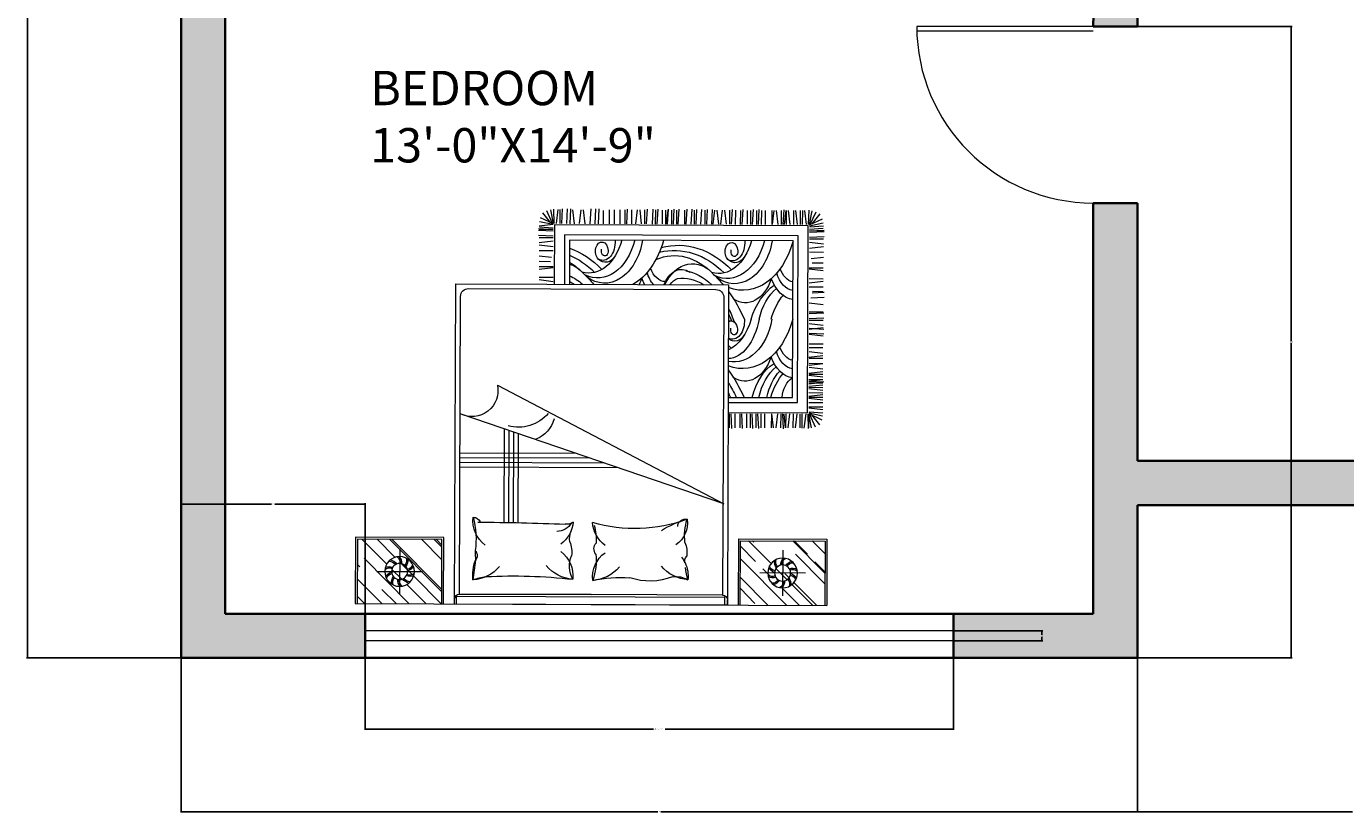
# Model space of a CAD drawing. Units: inches. Extents: x 1919 to 2461, y 2470 to 3159.
# Tile 1 of 6: x 1919 to 2188, y 2470 to 2630. Entities that reach past the tile are written whole.
import ezdxf

# ---------------------------------------------------------------- set-up
doc = ezdxf.new("R2010")
doc.units = ezdxf.units.IN
for name, color, linetype, lineweight in [('A-ANNO-DIMS', 2, 'Continuous', 18), ('A-AREA-IDEN', 7, 'Continuous', 18), ('A-DOOR', 3, 'Continuous', 18), ('A-FURN', 8, 'Continuous', 18), ('A-GLAZ', 4, 'Continuous', 18), ('A-WALL', 7, 'Continuous', 35), ('A-WALL-PATT', 252, 'Continuous', 13)]:
    doc.layers.add(name, color=color, linetype=linetype, lineweight=lineweight)
doc.styles.get("Standard").update_dxf_attribs({"font": 'arial.ttf'})
doc.dimstyles.get("Standard").update_dxf_attribs({"dimtxt": 0.18, "dimasz": 0.18, "dimexe": 0.18, "dimexo": 0.0625, "dimgap": 0.09, "dimtad": 0, "dimtih": 1, "dimtoh": 1, "dimdec": 4, "dimzin": 0, "dimdsep": 46, "dimtxsty": 'Standard', "dimcen": 0.09, "dimadec": 0, "dimazin": 0, "dimtfac": 1, "dimtdec": 4, "dimtofl": 0, "dimtmove": 0, "dimatfit": 3, "dimfxl": 1, "dimtolj": 1, "dimtzin": 0, "dimarcsym": 0})

# ---------------------------------------------------------------- blocks, each defined once
blk = doc.blocks.new('A$C64B41DC1')
for p, q in [((0, 2.5079), (2.9903, 2.5079)), ((0, 2.0879), (0, 2.5079)), ((0.012, 2.4618), (0.0581, 2.5079)), ((0.012, 2.3515), (0.1684, 2.5079)), ((0.012, 2.0999), (0.012, 2.5079)), ((0.0543, 2.2213), (0.3409, 2.5079)), ((0.1689, 2.4179), (0.2589, 2.5079)), ((0.2157, 2.0999), (0.548, 2.4322)), ((0.2804, 2.1597), (0.2804, 2.4481)), ((0.3265, 2.386), (0.4484, 2.5079)), ((0.3699, 2.3332), (0.5445, 2.5079)), ((0.548, 2.5079), (0.548, 2.0999)), ((0.56, 2.5079), (0.56, 2.0879)), ((0.6301, 2.5079), (0.6301, 0.4779)), ((0.6401, 2.461), (0.6401, 2.5079)), ((0.6401, 2.5079), (2.344, 2.5079)), ((2.344, 2.461), (0.6401, 2.461)), ((0.6601, 2.4461), (1.4951, 2.4461)), ((0.6601, 2.4461), (0.6601, 0.5579)), ((1.4951, 2.4461), (0.6697, 2.4461)), ((2.3301, 2.4461), (1.4951, 2.4461)), ((2.3301, 0.5579), (2.3301, 2.4461)), ((2.344, 2.5079), (2.3601, 2.5079)), ((2.344, 2.5079), (2.344, 2.461)), ((2.3601, 2.5079), (2.3601, 2.4761)), ((2.3601, 0.4779), (2.3601, 2.5079)), ((2.4303, 2.5079), (2.4303, 2.0879)), ((2.4423, 2.5079), (2.4423, 2.0999)), ((2.4423, 2.3333), (2.6169, 2.5079)), ((2.4423, 2.2145), (2.7357, 2.5079)), ((2.4423, 2.404), (2.5354, 2.4971)), ((2.705, 2.398), (2.8149, 2.5079)), ((2.7099, 2.1597), (2.7099, 2.4481)), ((2.7691, 2.3772), (2.8998, 2.5079)), ((2.7819, 2.3646), (2.9252, 2.5079)), ((2.9783, 2.0999), (2.9783, 2.5079)), ((2.9903, 2.0879), (2.9903, 2.5079)), ((0.2299, 2.0999), (0.548, 2.418)), ((0.2311, 2.2906), (0.2937, 2.3532)), ((2.6674, 2.2756), (2.7382, 2.3464)), ((2.7914, 2.1846), (2.9783, 2.3715)), ((0.012, 2.261), (0.0275, 2.2765)), ((0.1362, 2.3039), (0.4246, 2.3039)), ((0.2905, 2.2539), (0.3304, 2.2938)), ((0.3405, 2.3039), (0.3605, 2.3238)), ((2.8541, 2.3039), (2.5657, 2.3039)), ((2.5849, 2.2779), (2.6158, 2.3088)), ((2.6158, 2.3088), (2.6313, 2.3243)), ((2.7249, 2.3076), (2.7512, 2.3339)), ((2.7746, 2.0999), (2.9783, 2.3036)), ((2.9144, 2.2312), (2.9783, 2.2951)), ((0.0404, 2.0999), (0.1982, 2.2578)), ((0.1365, 2.0999), (0.251, 2.2144)), ((0.4194, 2.0999), (0.548, 2.2285)), ((2.4423, 2.1353), (2.5382, 2.2312)), ((2.4918, 2.0999), (2.6366, 2.2447)), ((2.7831, 2.0999), (2.8678, 2.1846)), ((2.8962, 2.0999), (2.9783, 2.182)), ((0.548, 2.0999), (0.012, 2.0999)), ((0.4986, 2.0999), (0.548, 2.1493)), ((0.5127, 2.0999), (0.548, 2.1352)), ((2.4423, 2.0999), (2.9783, 2.0999)), ((2.5172, 2.0999), (2.5269, 2.1096)), ((0.56, 2.0879), (0, 2.0879)), ((2.4303, 2.0879), (2.9903, 2.0879)), ((0.9415, 1.9902), (0.9415, 1.3975)), ((0.9715, 1.9906), (0.9715, 1.4076)), ((1.0015, 1.991), (1.0015, 1.4177)), ((1.0315, 1.9916), (1.0315, 1.4279)), ((2.3349, 1.8678), (0.6613, 1.3029)), ((0.8956, 1.1191), (2.3349, 1.8678)), ((1.6636, 1.6412), (0.6601, 1.6412)), ((1.5748, 1.6112), (0.6601, 1.6112)), ((2.3665, 1.295), (2.3665, 1.3839)), ((2.377, 1.295), (2.3822, 1.3891)), ((2.4032, 1.295), (2.4032, 1.3839)), ((2.4346, 1.295), (2.4346, 1.3839)), ((2.4451, 1.295), (2.4503, 1.3891)), ((2.4774, 1.2957), (2.4774, 1.3837)), ((2.5, 1.295), (2.5, 1.3839)), ((2.5105, 1.295), (2.5157, 1.3891)), ((2.5367, 1.295), (2.5367, 1.3839)), ((2.5471, 1.295), (2.5524, 1.3891)), ((2.5681, 1.295), (2.5681, 1.3839)), ((2.5918, 1.295), (2.5918, 1.3839)), ((2.6346, 1.2957), (2.6346, 1.3837)), ((2.6362, 1.2957), (2.6467, 1.3839)), ((2.6729, 1.295), (2.6624, 1.3839)), ((2.6938, 1.295), (2.6938, 1.3839)), ((2.7043, 1.295), (2.7095, 1.3891)), ((2.7127, 1.2957), (2.7232, 1.3839)), ((2.7253, 1.295), (2.7253, 1.3839)), ((2.7494, 1.295), (2.7389, 1.3839)), ((2.7718, 1.295), (2.7718, 1.3839)), ((2.7959, 1.295), (2.7854, 1.3839)), ((2.8146, 1.2957), (2.8146, 1.3837)), ((2.8146, 1.2957), (2.8146, 1.3837)), ((2.8282, 1.295), (2.8282, 1.3839)), ((2.8282, 1.295), (2.8282, 1.3839)), ((2.8523, 1.295), (2.8418, 1.3839)), ((2.8523, 1.295), (2.8418, 1.3839)), ((2.8653, 1.2966), (2.8688, 1.3861)), ((2.8711, 1.2957), (2.8711, 1.3837)), ((2.8711, 1.2957), (2.8875, 1.3822)), ((2.8765, 1.2958), (2.9132, 1.3758)), ((2.8893, 1.3011), (2.9394, 1.3636)), ((2.3601, 1.2873), (2.8639, 1.2873)), ((2.8639, 1.2873), (2.8639, 0.1018)), ((2.8713, 1.2927), (2.954, 1.3315)), ((2.8716, 1.2565), (2.9605, 1.2669)), ((2.8717, 1.2884), (2.9588, 1.3058)), ((2.8744, 1.2817), (2.9603, 1.2869)), ((2.3601, 1.2233), (2.7999, 1.2233)), ((2.3601, 1.1913), (2.7679, 1.1912)), ((2.7679, 1.1912), (2.7679, 0.1978)), ((2.7999, 1.2233), (2.7999, 0.1658)), ((2.8716, 1.2212), (2.9605, 1.2212)), ((2.8716, 1.1947), (2.9605, 1.2052)), ((2.8716, 1.181), (2.9605, 1.1705)), ((2.8723, 1.2489), (2.9603, 1.2489)), ((2.8723, 1.1872), (2.9603, 1.1872)), ((2.8716, 1.1595), (2.9605, 1.1595)), ((2.8716, 1.133), (2.9605, 1.1435)), ((2.8716, 1.1193), (2.9605, 1.1088)), ((2.8716, 1.1035), (2.9605, 1.093)), ((2.8716, 1.0965), (2.9605, 1.0965)), ((2.8716, 1.086), (2.9657, 1.0913)), ((2.8723, 1.1255), (2.9603, 1.1255)), ((2.8716, 1.0756), (2.9605, 1.0756)), ((2.8716, 1.0491), (2.9605, 1.0596)), ((2.8716, 1.0354), (2.9605, 1.0249)), ((2.8723, 1.0858), (2.9605, 1.0753)), ((2.8723, 1.0416), (2.9603, 1.0416)), ((2.8723, 0.9987), (2.9605, 1.0092)), ((2.8716, 0.9346), (2.9605, 0.9241)), ((2.8723, 0.985), (2.9605, 0.9745)), ((2.8723, 0.9735), (2.9603, 0.9735)), ((2.8723, 0.9408), (2.9603, 0.9408)), ((2.8723, 0.8979), (2.9605, 0.9084)), ((2.8723, 0.8726), (2.9603, 0.8726)), ((2.8723, 0.8505), (2.9603, 0.8505)), ((2.8716, 0.7885), (2.9605, 0.799)), ((2.8716, 0.7818), (2.9657, 0.787)), ((2.8716, 0.7503), (2.9657, 0.7556)), ((2.8723, 0.7571), (2.9605, 0.7466)), ((2.8716, 0.7204), (2.9605, 0.7309)), ((2.8716, 0.6995), (2.9605, 0.6995)), ((2.8716, 0.689), (2.9657, 0.6838)), ((2.8716, 0.6576), (2.9657, 0.6523)), ((2.8716, 0.6471), (2.9605, 0.6471)), ((2.8716, 0.5903), (2.9605, 0.6007)), ((0.7101, 0.5079), (2.2801, 0.5079)), ((2.882, 0.5582), (2.9657, 0.5536)), ((2.8909, 0.5263), (2.9657, 0.5222)), ((2.8928, 0.5169), (2.9605, 0.5169)), ((0.6301, 0.4779), (2.3601, 0.4779)), ((1.2465, 0.4625), (1.1576, 0.452)), ((1.2465, 0.4365), (1.1577, 0.4365)), ((1.2542, 0.1018), (1.2542, 0.4779)), ((1.3182, 0.1658), (1.3182, 0.4779)), ((1.3502, 0.1978), (1.3502, 0.4779)), ((2.8716, 0.4877), (2.9603, 0.4877)), ((2.8716, 0.4625), (2.9605, 0.452)), ((2.8716, 0.4365), (2.9603, 0.4365)), ((1.2465, 0.3746), (1.1576, 0.3851)), ((1.2465, 0.3684), (1.1577, 0.3684)), ((1.2285, 0.3357), (1.1577, 0.3357)), ((2.8716, 0.3746), (2.9605, 0.3851)), ((2.8716, 0.3684), (2.9603, 0.3684)), ((2.8896, 0.3357), (2.9603, 0.3357)), ((1.2355, 0.3092), (1.1576, 0.3)), ((1.2457, 0.2676), (1.1577, 0.2676)), ((2.8723, 0.2676), (2.9603, 0.2676)), ((2.8826, 0.3092), (2.9605, 0.3)), ((1.2465, 0.1742), (1.1524, 0.169)), ((1.2457, 0.2423), (1.1576, 0.2319)), ((1.2465, 0.2057), (1.1576, 0.2161)), ((1.2465, 0.1847), (1.1576, 0.1847)), ((2.7679, 0.1978), (1.3502, 0.1978)), ((2.8716, 0.2057), (2.9605, 0.2161)), ((2.8716, 0.1847), (2.9605, 0.1847)), ((2.8716, 0.1742), (2.9657, 0.169)), ((2.8723, 0.2423), (2.9605, 0.2319)), ((1.2465, 0.1428), (1.1524, 0.1376)), ((1.2465, 0.1334), (1.1524, 0.1281)), ((1.2465, 0.1323), (1.1576, 0.1323)), ((1.2465, 0.1323), (1.1576, 0.1323)), ((1.2465, 0.1), (1.1576, 0.1105)), ((1.2465, 0.1229), (1.1588, 0.1168)), ((1.2464, 0.1007), (1.1592, 0.0833)), ((1.2468, 0.0964), (1.1641, 0.0576)), ((1.2288, 0.088), (1.1787, 0.0255)), ((1.2415, 0.0933), (1.2049, 0.0133)), ((1.247, 0.0934), (1.2306, 0.0069)), ((1.2527, 0.0925), (1.2493, 0.003)), ((2.8639, 0.1018), (1.2542, 0.1018)), ((1.2658, 0.0941), (1.2762, 0.0052)), ((1.2899, 0.0941), (1.2899, 0.0052)), ((1.2999, 0.0941), (1.3051, 0)), ((2.7999, 0.1658), (1.3182, 0.1658)), ((1.3313, 0.0941), (1.3365, 0)), ((1.3523, 0.0941), (1.3575, 0)), ((1.3804, 0.0941), (1.3699, 0.0052)), ((1.4119, 0.0934), (1.4223, 0.0052)), ((1.4485, 0.0941), (1.438, 0.0052)), ((1.48, 0.0941), (1.4852, 0)), ((1.5114, 0.0941), (1.5166, 0)), ((1.5323, 0.0941), (1.5376, 0)), ((1.5638, 0.0941), (1.5638, 0.0105)), ((1.6021, 0.0941), (1.6021, 0.0052)), ((1.6336, 0.0941), (1.6336, 0.0052)), ((1.6702, 0.0941), (1.6702, 0.0052)), ((1.7017, 0.0941), (1.7017, 0.0052)), ((1.7122, 0.0941), (1.7174, 0)), ((1.7445, 0.0934), (1.7445, 0.0054)), ((1.7698, 0.0934), (1.7803, 0.0052)), ((1.8065, 0.0941), (1.796, 0.0052)), ((1.8274, 0.0941), (1.8274, 0.0052)), ((1.8379, 0.0941), (1.8431, 0)), ((1.8746, 0.0941), (1.8798, 0)), ((1.8955, 0.0941), (1.8955, 0.0052)), ((1.906, 0.0941), (1.9113, 0)), ((1.9384, 0.0934), (1.9384, 0.0054)), ((1.9609, 0.0941), (1.9609, 0.0052)), ((1.9636, 0.0934), (1.9741, 0.0052)), ((1.9714, 0.0941), (1.9766, 0)), ((1.9976, 0.0941), (1.9976, 0.0052)), ((2.0081, 0.0941), (2.0133, 0)), ((2.029, 0.0941), (2.029, 0.0052)), ((2.0395, 0.0941), (2.0447, 0)), ((2.0797, 0.0941), (2.0797, 0.0052)), ((2.0902, 0.0941), (2.0954, 0)), ((2.1216, 0.0941), (2.1269, 0)), ((2.1412, 0.0941), (2.1412, 0.0052)), ((2.1517, 0.0941), (2.1569, 0)), ((2.1831, 0.0941), (2.1884, 0)), ((2.2093, 0.0941), (2.2093, 0.0052)), ((2.2198, 0.0941), (2.225, 0)), ((2.2512, 0.0941), (2.2565, 0)), ((2.2603, 0.0934), (2.2707, 0.0052)), ((2.2969, 0.0941), (2.2864, 0.0052)), ((2.3089, 0.0934), (2.3193, 0.0052)), ((2.3455, 0.0941), (2.3351, 0.0052)), ((2.3665, 0.0941), (2.3665, 0.0052)), ((2.377, 0.0941), (2.3822, 0)), ((2.4032, 0.0941), (2.4032, 0.0052)), ((2.4346, 0.0941), (2.4346, 0.0052)), ((2.4451, 0.0941), (2.4503, 0)), ((2.4774, 0.0934), (2.4774, 0.0054)), ((2.5, 0.0941), (2.5, 0.0052)), ((2.5105, 0.0941), (2.5157, 0)), ((2.5367, 0.0941), (2.5367, 0.0052)), ((2.5471, 0.0941), (2.5524, 0)), ((2.5681, 0.0941), (2.5681, 0.0052)), ((2.5918, 0.0941), (2.5918, 0.0052)), ((2.6346, 0.0934), (2.6346, 0.0054)), ((2.6362, 0.0934), (2.6467, 0.0052)), ((2.6729, 0.0941), (2.6624, 0.0052)), ((2.6938, 0.0941), (2.6938, 0.0052)), ((2.7043, 0.0941), (2.7095, 0)), ((2.7127, 0.0934), (2.7232, 0.0052)), ((2.7253, 0.0941), (2.7253, 0.0052)), ((2.7494, 0.0941), (2.7389, 0.0052)), ((2.7718, 0.0941), (2.7718, 0.0052)), ((2.7959, 0.0941), (2.7854, 0.0052)), ((2.8146, 0.0934), (2.8146, 0.0054)), ((2.8282, 0.0941), (2.8282, 0.0052)), ((2.8523, 0.0941), (2.8418, 0.0052)), ((2.8653, 0.0925), (2.8688, 0.003)), ((2.8711, 0.0934), (2.8875, 0.0069)), ((2.8713, 0.0964), (2.954, 0.0576)), ((2.8716, 0.1428), (2.9657, 0.1376)), ((2.8716, 0.1334), (2.9657, 0.1281)), ((2.8716, 0.1323), (2.9605, 0.1323)), ((2.8716, 0.1229), (2.9593, 0.1168)), ((2.8717, 0.1007), (2.9588, 0.0833)), ((2.8744, 0.1074), (2.9603, 0.1022)), ((2.8765, 0.0933), (2.9132, 0.0133)), ((2.8893, 0.088), (2.9394, 0.0255))]:
    blk.add_line(p, q)
at = {"ltscale": 10}
for p, q in [((1.4859, 1.5812), (0.6601, 1.5812)), ((1.397, 1.5512), (0.6601, 1.5512))]:
    blk.add_line(p, q, dxfattribs=at)
for centre, radius in [((0.2804, 2.3039), 0.0942), ((0.2804, 2.3039), 0.051), ((2.7099, 2.3039), 0.0942), ((2.7099, 2.3039), 0.051)]:
    blk.add_circle(centre, radius)
for centre, radius, start, end in [((0.6601, 2.4761), 0.03, 180, 270), ((2.3301, 2.4761), 0.03, 270, 0), ((0.2417, 2.3614), 0.0462, 196.30017, 256.53802), ((0.2887, 2.3745), 0.0605, 172.17003, 218.48975), ((0.2828, 2.3731), 0.0462, 160.30017, 220.53802), ((0.3286, 2.3561), 0.0605, 136.17003, 182.48975), ((0.3231, 2.3585), 0.0462, 124.30017, 184.53802), ((0.3501, 2.3178), 0.0605, 100.17003, 146.48975), ((0.347, 2.323), 0.0462, 88.30017, 148.53802), ((1.0526, 2.3302), 0.3085, 175.30484, 198.69419), ((-0.8702, 2.0941), 1.6364, 4.80985, 9.18918), ((0.8579, 2.6278), 0.2948, 247.51785, 264.26696), ((0.728, 2.111), 0.245, 40.4189, 85.9871), ((1.0164, 5.7096), 3.3803, 266.81337, 276.16021), ((1.3963, 2.1044), 0.245, 94.0129, 139.5811), ((1.1858, 2.3288), 0.1943, 306.5711, 5.88998), ((1.5348, 2.2652), 0.1767, 151.77364, 201.69827), ((1.6986, 2.3355), 0.1943, 174.11002, 233.4289), ((1.1481, 2.2311), 0.3783, 353.49469, 19.18669), ((1.6871, 3.192), 0.8561, 257.74383, 273.62843), ((1.4882, 2.111), 0.245, 40.4189, 85.9871), ((1.8674, 1.9709), 0.3878, 68.20259, 108.9817), ((2.1269, 2.1044), 0.245, 94.0129, 139.5811), ((2.0342, 2.4856), 0.1563, 261.59582, 298.90918), ((1.9165, 2.3288), 0.1943, 333.73715, 5.88998), ((2.6058, 2.2028), 0.517, 163.60457, 172.3273), ((2.6433, 2.323), 0.0462, 31.46198, 91.69983), ((2.6402, 2.3178), 0.0605, 33.51025, 79.82997), ((2.6672, 2.3585), 0.0462, 355.46198, 55.69983), ((2.6617, 2.3561), 0.0605, 357.51025, 43.82997), ((2.7075, 2.3731), 0.0462, 319.46198, 19.69983), ((2.7016, 2.3745), 0.0605, 321.51025, 7.82997), ((2.7486, 2.3614), 0.0462, 283.46198, 343.69983), ((0.2153, 2.3276), 0.0462, 232.30017, 292.53802), ((0.2158, 2.3336), 0.0605, 244.17003, 290.48975), ((0.2457, 2.3659), 0.0605, 208.17003, 254.48975), ((0.2138, 2.2848), 0.0462, 268.30017, 328.53802), ((0.2779, 2.2347), 0.0462, 340.30017, 40.53802), ((0.272, 2.2333), 0.0605, 352.17003, 38.48975), ((0.3449, 2.2742), 0.0605, 64.17003, 110.48975), ((0.3455, 2.2802), 0.0462, 52.30017, 112.53802), ((0.3191, 2.2464), 0.0462, 16.30017, 76.53802), ((0.3151, 2.2419), 0.0605, 28.17003, 74.48975), ((2.6448, 2.2802), 0.0462, 67.46198, 127.69983), ((2.6454, 2.2742), 0.0605, 69.51025, 115.82997), ((2.6752, 2.2419), 0.0605, 105.51025, 151.82997), ((2.6712, 2.2464), 0.0462, 103.46198, 163.69983), ((2.7182, 2.2333), 0.0605, 141.51025, 187.82997), ((2.7123, 2.2347), 0.0462, 139.46198, 199.69983), ((2.7765, 2.2848), 0.0462, 211.46198, 271.69983), ((2.7744, 2.3336), 0.0605, 249.51025, 295.82997), ((2.775, 2.3276), 0.0462, 247.46198, 307.69983), ((2.7446, 2.3659), 0.0605, 285.51025, 331.82997), ((0.2107, 2.29), 0.0605, 280.17003, 326.48975), ((0.2377, 2.2493), 0.0462, 304.30017, 4.53802), ((0.2322, 2.2517), 0.0605, 316.17003, 2.48975), ((0.7274, 2.2013), 0.0446, 314.4736, 42.17134), ((-1.6008, 2.277), 2.3618, 357.39054, 358.88764), ((1.204, 2.1778), 0.1681, 337.01697, 7.53676), ((1.5671, 2.1546), 0.0547, 142.08329, 220.902), ((1.9165, 2.3288), 0.1943, 320.94042, 333.73715), ((2.1347, 2.2313), 0.0459, 165.35061, 223.26844), ((1.9346, 2.1778), 0.1681, 337.01697, 7.53676), ((2.7581, 2.2517), 0.0605, 177.51025, 223.82997), ((2.7526, 2.2493), 0.0462, 175.46198, 235.69983), ((2.7796, 2.29), 0.0605, 213.51025, 259.82997), ((0.9385, 1.978), 0.1943, 126.5711, 185.88998), ((0.2688, 2.0945), 0.4956, 344.0243, 8.70709), ((1.1858, 1.9714), 0.1943, 4.31813, 53.4289), ((1.5415, 2.0969), 0.1834, 175.22328, 196.23004), ((1.7059, 1.9714), 0.204, 127.11975, 175.09005), ((1.1965, 2.0983), 0.3299, 343.79543, 3.55541), ((1.9394, 1.991), 0.1651, 351.26213, 55.75721), ((2.4617, 2.0719), 0.3745, 173.82958, 196.4356), ((1.2687, 1.9248), 0.1223, 33.62799, 86.47438), ((1.7676, 1.0629), 0.9631, 69.65065, 105.96307), ((2.2748, 2.5795), 0.6373, 238.34989, 254.31375), ((2.0911, 2.0123), 0.0478, 179.77267, 283.80184), ((0.7417, 2.0149), 0.057, 273.47085, 328.54118), ((0.728, 2.2025), 0.245, 274.0129, 278.34166), ((0.7246, 18.8439), 16.8552, 270.17399, 272.05214), ((1.3401, 1.9404), 0.0603, 49.09906, 101.37023), ((1.0747, 1.2871), 0.1871, 14.1863, 69.12121), ((1.0274, 1.1334), 0.2527, 40.62904, 104.37123), ((0.7347, 1.1553), 0.1649, 347.31088, 116.44537), ((0.7101, 0.5579), 0.05, 180, 270), ((2.2801, 0.5579), 0.05, 270, 0)]:
    blk.add_arc(centre, radius, start, end)
for centre, major_axis, ratio, start_param, end_param in [((1.9938, 1.6262), (0, -0.7531), 0.68, 0.797284, 0.954936), ((2.0643, 1.466), (0, -0.5322), 0.68, 7.239912, 7.311536), ((1.9052, 1.7397), (0, -0.9842), 0.68, 0.74745, 0.979724), ((2.7455, 1.3081), (0, 0.3614), 0.68, 1.900046, 2.742661), ((2.7868, 1.3081), (0, 0.3614), 0.68, 1.900046, 2.614747), ((2.8372, 1.3081), (0, 0.3614), 0.68, 1.900046, 2.479658), ((2.8607, 1.3211), (0, 0.3614), 0.68, 1.938265, 2.479658), ((2.8057, 1.2079), (0, -0.1524), 0.68, 4.821745, 5.895886), ((2.4665, 0.8216), (0, -0.2664), 0.68, 2.006169, 3.565187), ((2.4513, 0.5069), (0, 0.502), 0.68, 5.095327, 6.553458), ((2.7862, 0.8069), (0, -0.2615), 0.68, 3.244645, 4.205018), ((2.7784, 0.8289), (0, -0.1802), 0.68, 3.227058, 4.318474), ((2.396, 0.6032), (0, 0.3641), 0.68, -1.3172, 0.145284), ((2.3507, 0.5642), (0.0073, 0.3819), 0.56205, -1.21172, -0.009991), ((2.7821, 0.7971), (0, -0.1589), 0.68, 3.272942, 4.229533), ((2.2964, 0.5771), (0, -0.3263), 0.68, 1.938944, 2.850232), ((2.0403, 1.6015), (0, -0.8763), 0.68, 6.849801, 6.887077), ((2.4005, 0.7132), (0, -0.1214), 0.68, 2.284368, 3.652258), ((2.3834, 0.7081), (0, 0.1147), 0.68, 4.593909, 6.585576), ((2.3774, 0.7653), (0, -0.0593), 0.68, 5.841311, 7.755362), ((2.3961, 0.7628), (0, -0.0317), 0.68, 1.462497, 5.046281), ((1.9938, 1.1295), (-0.0678, 0.7439), 0.610498, 3.917146, 4.063997), ((2.0643, 0.9693), (0, -0.5322), 0.68, 7.239912, 7.336618), ((1.9052, 1.243), (0, -0.9842), 0.68, 0.74745, 0.979724), ((2.7455, 0.8114), (-0.0599, 0.3735), 0.695517, 1.775813, 2.548612), ((2.7868, 0.8114), (0, 0.3614), 0.68, 1.900046, 2.614747), ((2.8607, 0.8243), (0, 0.3614), 0.68, 1.938265, 2.479658), ((2.4665, 0.3249), (0, -0.2664), 0.68, 2.006169, 3.565187), ((2.4513, 0.0102), (0, 0.502), 0.68, 5.095327, 6.553458), ((2.7862, 0.3102), (0, -0.2615), 0.68, 3.244645, 4.205018), ((2.7784, 0.3322), (0, -0.1802), 0.68, 3.227058, 4.318474), ((1.242, 0.9693), (0, -0.5322), 0.68, 6.586764, 6.677612), ((1.1714, 1.1295), (-0.1157, 0.7241), 0.59432, 3.291697, 3.50733), ((1.474, 0.0804), (0, -0.3263), 0.68, 1.938944, 3.339184), ((1.0828, 1.243), (0, -0.9842), 0.68, 0.565948, 0.680366), ((1.5283, 0.0674), (0, -0.3703), 0.68, 1.930561, 3.464283), ((1.5736, 0.1065), (0, 0.3641), 0.68, -1.3172, 0.476403), ((1.6289, 0.0102), (0, 0.502), 0.68, 6.655152, 6.661293), ((1.6289, 0.0102), (0, 0.502), 0.68, 5.095327, 5.911219), ((1.6442, 0.3249), (0, -0.2664), 0.68, 2.006169, 2.182797), ((1.9638, 0.3102), (0, -0.2615), 0.68, 4.015924, 4.205018), ((1.956, 0.3322), (0, -0.1802), 0.68, 3.770744, 4.318474), ((1.9597, 0.3004), (0, -0.1589), 0.68, 3.14258, 4.229533), ((2.0606, 0.5616), (0, -0.1803), 0.68, 5.194792, 5.929328), ((2.0606, 0.5616), (0, -0.1803), 0.68, 5.194792, 6.723255), ((2.1315, 0.6603), (0, -0.3155), 0.68, 5.328638, 6.949396), ((2.0549, 0.5656), (0, -0.1303), 0.68, 5.450951, 6.054641), ((2.0643, 0.9693), (0, -0.5322), 0.68, 6.20013, 6.677612), ((1.9938, 1.1295), (-0.0678, 0.7439), 0.610498, 3.199135, 3.592282), ((2.2964, 0.0804), (0, -0.3263), 0.68, 1.938944, 3.339184), ((1.9052, 1.243), (0, -0.9842), 0.68, 0.565948, 0.680366), ((2.3507, 0.0674), (0, -0.3703), 0.68, 1.930561, 3.464283), ((2.396, 0.1065), (0, 0.3641), 0.68, -1.3172, 0.476403), ((2.4513, 0.0102), (0, 0.502), 0.68, 6.655152, 6.661293), ((2.7821, 0.3004), (0, -0.1589), 0.68, 3.272942, 4.229533), ((1.1933, 0.9181), (0, -0.624), 0.68, 0.378672, 0.625379), ((1.3091, 0.6603), (0, -0.3155), 0.68, 6.475719, 6.949396), ((1.1911, 1.1066), (0, 0.8458), 0.68, 3.421828, 3.728616), ((1.2179, 1.1047), (0, -0.8763), 0.68, 6.507006, 6.887077), ((1.5781, 0.2165), (0, -0.1214), 0.68, 2.284368, 3.726131), ((2.0157, 0.9181), (0, -0.624), 0.68, -0.280078, 0.625379), ((2.0135, 1.1066), (0, 0.8458), 0.68, 2.978727, 3.728616), ((2.0403, 1.1047), (0, -0.8763), 0.68, 6.099302, 6.887077), ((2.4005, 0.2165), (0, -0.1214), 0.68, 2.284368, 3.726131), ((1.555, 0.2685), (0, -0.0593), 0.68, 3.732151, 7.755362), ((1.561, 0.2114), (0, 0.1147), 0.68, 4.593909, 6.647252), ((1.5737, 0.2661), (0, -0.0317), 0.68, 1.462497, 5.046281), ((2.3774, 0.2685), (0, -0.0593), 0.68, 3.732151, 7.755362), ((2.3834, 0.2114), (0, 0.1147), 0.68, 4.593909, 6.647252), ((2.3961, 0.2661), (0, -0.0317), 0.68, 1.462497, 5.046281)]:
    blk.add_ellipse(centre, major_axis=major_axis, ratio=ratio, start_param=start_param, end_param=end_param)
blk = doc.blocks.new('WIN-GLAZ-120IN')
for p, q in [((120, 0), (0, 0)), ((120, -2), (0, -2))]:
    blk.add_line(p, q)
blk = doc.blocks.new('*D17')
at = {"layer": 'A-ANNO-DIMS', "color": 0, "lineweight": -2, "transparency": 16777216}
for p, q in [((1987.82, 2505.11), (1987.82, 2486.99)), ((2107.82, 2505.11), (2107.82, 2486.99)), ((1988, 2487.17), (2046.63, 2487.17)), ((2107.64, 2487.17), (2049, 2487.17))]:
    blk.add_line(p, q, dxfattribs=at)
at = {"layer": 'A-ANNO-DIMS', "color": 0, "transparency": 16777216}
for points in [[(1988, 2487.2), (1988, 2487.14), (1987.82, 2487.17)], [(2107.64, 2487.2), (2107.64, 2487.14), (2107.82, 2487.17)]]:
    blk.add_solid(points, dxfattribs=at)
at = {"layer": 'Defpoints', "color": 0, "transparency": 16777216}
for p in [(1987.82, 2505.17), (2107.82, 2505.17), (2107.82, 2487.17)]:
    blk.add_point(p, dxfattribs=at)
at = {"layer": 'A-ANNO-DIMS', "color": 0, "transparency": 16777216, "insert": (2047.82, 2487.17), "char_height": 0.18, "attachment_point": 5}
blk.add_mtext('\\A1;WINDOW 120 TYP.', dxfattribs=at)
blk = doc.blocks.new('*D18')
at = {"layer": 'A-ANNO-DIMS', "color": 0, "lineweight": -2, "transparency": 16777216}
for p, q in [((2107.88, 2507.17), (2126, 2507.17)), ((2107.88, 2505.17), (2126, 2505.17)), ((2125.82, 2506.99), (2125.82, 2506.35)), ((2125.82, 2505.35), (2125.82, 2505.99))]:
    blk.add_line(p, q, dxfattribs=at)
at = {"layer": 'A-ANNO-DIMS', "color": 0, "transparency": 16777216}
for points in [[(2125.79, 2506.99), (2125.85, 2506.99), (2125.82, 2507.17)], [(2125.79, 2505.35), (2125.85, 2505.35), (2125.82, 2505.17)]]:
    blk.add_solid(points, dxfattribs=at)
at = {"layer": 'Defpoints', "color": 0, "transparency": 16777216}
for p in [(2107.82, 2507.17), (2125.82, 2507.17), (2107.82, 2505.17)]:
    blk.add_point(p, dxfattribs=at)
at = {"layer": 'A-ANNO-DIMS', "color": 0, "transparency": 16777216, "insert": (2125.82, 2506.17), "char_height": 0.18, "attachment_point": 5}
blk.add_mtext('\\A1;2 TYP.', dxfattribs=at)
blk = doc.blocks.new('*D24')
at = {"layer": 'A-ANNO-DIMS', "color": 0, "lineweight": -2, "transparency": 16777216}
for p, q in [((2004.25, 3127.67), (1918.78, 3127.67)), ((1918.96, 3127.49), (1918.96, 2814.85)), ((1918.96, 2501.85), (1918.96, 2814.49)), ((1950.25, 2501.67), (1918.78, 2501.67))]:
    blk.add_line(p, q, dxfattribs=at)
at = {"layer": 'A-ANNO-DIMS', "color": 0, "transparency": 16777216}
for points in [[(1918.93, 3127.49), (1918.99, 3127.49), (1918.96, 3127.67)], [(1918.93, 2501.85), (1918.99, 2501.85), (1918.96, 2501.67)]]:
    blk.add_solid(points, dxfattribs=at)
at = {"layer": 'Defpoints', "color": 0, "transparency": 16777216}
for p in [(1918.96, 3127.67), (2004.32, 3127.67), (1950.32, 2501.67)]:
    blk.add_point(p, dxfattribs=at)
at = {"layer": 'A-ANNO-DIMS', "color": 0, "transparency": 16777216, "insert": (1918.96, 2814.67), "char_height": 0.18, "attachment_point": 5}
blk.add_mtext('\\A1;626', dxfattribs=at)
blk = doc.blocks.new('*D32')
at = {"layer": 'A-ANNO-DIMS', "color": 0, "lineweight": -2, "transparency": 16777216}
for p, q in [((1950.32, 2501.73), (1950.32, 2533.21)), ((1950.5, 2533.03), (1968.74, 2533.03)), ((1987.64, 2533.03), (1969.39, 2533.03)), ((1987.82, 2501.73), (1987.82, 2533.21))]:
    blk.add_line(p, q, dxfattribs=at)
at = {"layer": 'A-ANNO-DIMS', "color": 0, "transparency": 16777216}
for points in [[(1950.5, 2533.06), (1950.5, 2533), (1950.32, 2533.03)], [(1987.64, 2533.06), (1987.64, 2533), (1987.82, 2533.03)]]:
    blk.add_solid(points, dxfattribs=at)
at = {"layer": 'Defpoints', "color": 0, "transparency": 16777216}
for p in [(1987.82, 2533.03), (1950.32, 2501.67), (1987.82, 2501.67)]:
    blk.add_point(p, dxfattribs=at)
at = {"layer": 'A-ANNO-DIMS', "color": 0, "transparency": 16777216, "insert": (1969.07, 2533.03), "char_height": 0.18, "attachment_point": 5}
blk.add_mtext('\\A1;37.5', dxfattribs=at)
blk = doc.blocks.new('*D33')
at = {"layer": 'A-ANNO-DIMS', "color": 0, "lineweight": -2, "transparency": 16777216}
for p, q in [((1950.32, 2501.61), (1950.32, 2470.14)), ((2145.32, 2501.61), (2145.32, 2470.14)), ((1950.5, 2470.32), (2047.53, 2470.32)), ((2145.14, 2470.32), (2048.1, 2470.32))]:
    blk.add_line(p, q, dxfattribs=at)
at = {"layer": 'A-ANNO-DIMS', "color": 0, "transparency": 16777216}
for points in [[(1950.5, 2470.35), (1950.5, 2470.29), (1950.32, 2470.32)], [(2145.14, 2470.35), (2145.14, 2470.29), (2145.32, 2470.32)]]:
    blk.add_solid(points, dxfattribs=at)
at = {"layer": 'Defpoints', "color": 0, "transparency": 16777216}
for p in [(1950.32, 2501.67), (2145.32, 2501.67), (2145.32, 2470.32)]:
    blk.add_point(p, dxfattribs=at)
at = {"layer": 'A-ANNO-DIMS', "color": 0, "transparency": 16777216, "insert": (2047.82, 2470.32), "char_height": 0.18, "attachment_point": 5}
blk.add_mtext('\\A1;195', dxfattribs=at)
blk = doc.blocks.new('*D34')
at = {"layer": 'A-ANNO-DIMS', "color": 0, "lineweight": -2, "transparency": 16777216}
for p, q in [((2145.32, 2532.77), (2145.32, 2470.14)), ((2233.88, 2532.77), (2233.88, 2470.14)), ((2145.5, 2470.32), (2189.2, 2470.32)), ((2233.7, 2470.32), (2189.99, 2470.32))]:
    blk.add_line(p, q, dxfattribs=at)
at = {"layer": 'A-ANNO-DIMS', "color": 0, "transparency": 16777216}
for points in [[(2145.5, 2470.35), (2145.5, 2470.29), (2145.32, 2470.32)], [(2233.7, 2470.35), (2233.7, 2470.29), (2233.88, 2470.32)]]:
    blk.add_solid(points, dxfattribs=at)
at = {"layer": 'Defpoints', "color": 0, "transparency": 16777216}
for p in [(2145.32, 2532.83), (2233.88, 2532.83), (2233.88, 2470.32)]:
    blk.add_point(p, dxfattribs=at)
at = {"layer": 'A-ANNO-DIMS', "color": 0, "transparency": 16777216, "insert": (2189.6, 2470.32), "char_height": 0.18, "attachment_point": 5}
blk.add_mtext('\\A1;88.56', dxfattribs=at)
blk = doc.blocks.new('*D35')
at = {"layer": 'A-ANNO-DIMS', "color": 0, "lineweight": -2, "transparency": 16777216}
for p, q in [((2145.38, 2630.39), (2176.85, 2630.39)), ((2176.67, 2630.21), (2176.67, 2566.21)), ((2176.67, 2501.85), (2176.67, 2565.85)), ((2145.38, 2501.67), (2176.85, 2501.67))]:
    blk.add_line(p, q, dxfattribs=at)
at = {"layer": 'A-ANNO-DIMS', "color": 0, "transparency": 16777216}
for points in [[(2176.64, 2630.21), (2176.7, 2630.21), (2176.67, 2630.39)], [(2176.64, 2501.85), (2176.7, 2501.85), (2176.67, 2501.67)]]:
    blk.add_solid(points, dxfattribs=at)
at = {"layer": 'Defpoints', "color": 0, "transparency": 16777216}
for p in [(2145.32, 2630.39), (2145.32, 2501.67), (2176.67, 2501.67)]:
    blk.add_point(p, dxfattribs=at)
at = {"layer": 'A-ANNO-DIMS', "color": 0, "transparency": 16777216, "insert": (2176.67, 2566.03), "char_height": 0.18, "attachment_point": 5}
blk.add_mtext('\\A1;128.72', dxfattribs=at)

msp = doc.modelspace()

# ---------------------------------------------------------------- hatches: boundary and pattern name
at = {"layer": 'A-WALL-PATT'}
h = msp.add_hatch(color=256, dxfattribs=at)
h.dxf.hatch_style = 1
h.paths.add_polyline_path([(1959.315, 2931.672), (2066.315, 2931.672), (2066.315, 2940.672), (2062.315, 2940.672), (2062.315, 3005.672), (2066.315, 3005.672), (2066.315, 3009.672), (2062.315, 3009.672), (2062.315, 3118.672), (2062.315, 3127.672), (2004.315, 3127.672), (2004.315, 3072.672), (1950.315, 3072.672), (1950.315, 3059.672), (1959.315, 3059.672), (1959.315, 3063.672), (2017.315, 3063.672), (2017.315, 3067.672), (2013.315, 3067.672), (2013.315, 3118.672), (2058.315, 3118.672), (2058.315, 3067.672), (2047.315, 3067.672), (2047.315, 3063.672), (2058.315, 3063.672), (2058.315, 2940.672), (1959.315, 2940.672), (1959.315, 2952.172), (1950.315, 2952.172), (1950.315, 2901.672), (1959.315, 2901.672)])
h.paths.add_polyline_path([(2120.315, 2791.672), (2145.315, 2791.672), (2145.315, 2795.672), (2124.315, 2795.672), (2124.315, 2803.3999), (2115.315, 2803.3999), (2115.315, 2799.3999), (2067.5871, 2751.672), (1959.315, 2751.672), (1959.315, 2781.672), (1950.315, 2781.672), (1950.315, 2718.672), (1959.315, 2718.672), (1959.315, 2742.672), (2067.315, 2742.672), (2067.315, 2670.672), (2063.315, 2670.672), (2063.315, 2666.672), (2143.3108, 2666.672, 0.09553844), (2136.315, 2630.3938), (2145.315, 2630.3938, -0.2455558), (2183.315, 2703.1037), (2183.315, 2713.8315, 0.15123975), (2145.0175, 2670.672), (2071.315, 2670.672), (2071.315, 2742.672)])
h.paths.add_polyline_path([(2124.315, 2931.672), (2232.315, 2931.672), (2232.315, 2940.672), (2228.315, 2940.672), (2228.315, 2964.672), (2219.315, 2964.672), (2219.315, 2940.672), (2138.315, 2940.672), (2138.315, 3005.672), (2185.315, 3005.672), (2185.315, 3009.672), (2138.315, 3009.672), (2138.315, 3118.672), (2138.315, 3127.672), (2086.315, 3127.672), (2086.315, 3118.672), (2134.315, 3118.672), (2134.315, 3009.672), (2096.315, 3009.672), (2096.315, 3005.672), (2134.315, 3005.672), (2134.315, 2940.672), (2096.315, 2940.672), (2096.315, 2931.672), (2115.315, 2931.672), (2115.315, 2839.3999), (2124.315, 2839.3999)])
h.paths.add_polyline_path([(2429.315, 3127.672), (2384.315, 3127.672), (2384.315, 3118.672), (2420.315, 3118.672), (2420.315, 2940.672), (2268.315, 2940.672), (2268.315, 2931.672), (2420.315, 2931.672), (2420.315, 2727.672), (2364.3064, 2727.672), (2317.4188, 2680.7844, 0.0404216), (2308.2227, 2693.5694), (2301.7735, 2687.2567, -0.63673951), (2233.8773, 2541.8315), (2145.315, 2541.8315), (2145.315, 2594.3938), (2136.315, 2594.3938), (2136.315, 2510.672), (2107.815, 2510.672), (2107.815, 2501.672), (2145.315, 2501.672), (2145.315, 2532.8315), (2233.8773, 2532.8315, 0.55190633), (2321.8781, 2672.5158), (2368.0343, 2718.672), (2429.315, 2718.672)])
h.paths.add_polyline_path([(2228.315, 3118.672), (2264.315, 3118.672), (2264.315, 3127.672), (2162.315, 3127.672), (2162.315, 3118.672), (2219.315, 3118.672), (2219.315, 3009.672), (2215.315, 3009.672), (2215.315, 3005.672), (2219.315, 3005.672), (2219.315, 2994.672), (2228.315, 2994.672)], flags=0)
h.paths.add_polyline_path([(1959.315, 2666.672), (2033.315, 2666.672), (2033.315, 2670.672), (1959.315, 2670.672), (1959.315, 2694.672), (1950.315, 2694.672), (1950.315, 2501.672), (1987.815, 2501.672), (1987.815, 2510.672), (1959.315, 2510.672)])

# ---------------------------------------------------------------- linework, layer by layer
at = {"layer": 'A-DOOR'}
for p, q in [((2136.315, 2630.3938), (2100.315, 2630.3938)), ((2136.315, 2629.3938), (2100.3289, 2629.3938))]:
    msp.add_line(p, q, dxfattribs=at)
msp.add_arc((2136.315, 2630.3938), 36, 180, 270, dxfattribs=at)
at = {"layer": 'A-WALL'}
for p, q in [((1950.315, 3023.672), (1950.315, 2501.672)), ((1959.315, 2666.672), (1959.315, 2510.672)), ((2145.315, 2630.3938), (2136.315, 2630.3938)), ((2136.315, 2594.3938), (2136.315, 2510.672)), ((2145.315, 2594.3938), (2136.315, 2594.3938)), ((2145.315, 2594.3938), (2145.315, 2541.8315)), ((2233.8773, 2541.8315), (2145.315, 2541.8315)), ((2233.8773, 2532.8315), (2145.315, 2532.8315)), ((2145.315, 2532.8315), (2145.315, 2501.672)), ((1959.315, 2510.672), (2136.315, 2510.672)), ((1987.815, 2510.672), (1987.815, 2501.672)), ((2107.815, 2510.672), (2107.815, 2501.672)), ((1950.315, 2501.672), (2145.315, 2501.672))]:
    msp.add_line(p, q, dxfattribs=at)
for radius, start in [(88.5623, 124.814645), (97.5623, 158.170458)]:
    msp.add_arc((2233.8773, 2630.3938), radius, start, 180, dxfattribs=at)

# ---------------------------------------------------------------- block references
at = {"layer": 'A-FURN', "xscale": -32.14386354378429, "yscale": 32.14386354378428, "zscale": 32.14386354378429, "rotation": 179.7714026471459}
msp.add_blockref('A$C64B41DC1', (1986.1509, 2593.379), dxfattribs=at)
at = {"layer": 'A-GLAZ'}
msp.add_blockref('WIN-GLAZ-120IN', (1987.815, 2507.172), dxfattribs=at)

# ---------------------------------------------------------------- texts
at = {"layer": 'A-AREA-IDEN', "insert": (1988.85, 2621.3325), "char_height": 7, "attachment_point": 1}
msp.add_mtext_dynamic_manual_height_columns('BEDROOM\\P13\'-0"X14\'-9"', width=121.344683, gutter_width=12.5, heights=[0], dxfattribs=at)

# ---------------------------------------------------------------- dimensions: what is measured, and where the dimension line sits
at = {"layer": 'A-ANNO-DIMS'}
for base, p1, p2, angle, override, picture, middle in [((1918.96, 3127.672), (1950.315, 2501.672), (2004.315, 3127.672), 90, {"dimdec": 0, "dimlfac": 1, "dimrnd": 0, "dimzin": 0, "dimdsep": 46, "dimlunit": 2}, '*D24', (1918.96, 2814.672)), ((2176.67, 2501.672), (2145.315, 2630.3938), (2145.315, 2501.672), 270, {"dimdec": 2, "dimlfac": 1, "dimrnd": 0, "dimzin": 0, "dimdsep": 46, "dimlunit": 2}, '*D35', (2176.67, 2566.0329))]:
    dim = msp.add_linear_dim(base=base, p1=p1, p2=p2, angle=angle, dimstyle='Standard', override=override, dxfattribs=at)
    dim.commit()
    dim.dimension.update_dxf_attribs({"geometry": picture, "text_midpoint": middle})
for base, p1, p2, override, picture, middle in [((1987.815, 2533.027), (1950.315, 2501.672), (1987.815, 2501.672), {"dimdec": 1, "dimlfac": 1, "dimrnd": 0, "dimzin": 0, "dimdsep": 46, "dimlunit": 2}, '*D32', (1969.065, 2533.027)), ((2233.8773, 2470.317), (2145.315, 2532.8315), (2233.8773, 2532.8315), {"dimdec": 2, "dimlfac": 1, "dimrnd": 0, "dimzin": 0, "dimdsep": 46, "dimlunit": 2}, '*D34', (2189.5962, 2470.317)), ((2145.315, 2470.317), (1950.315, 2501.672), (2145.315, 2501.672), {"dimdec": 0, "dimlfac": 1, "dimrnd": 0, "dimzin": 0, "dimdsep": 46, "dimlunit": 2}, '*D33', (2047.815, 2470.317))]:
    dim = msp.add_linear_dim(base=base, p1=p1, p2=p2, dimstyle='Standard', override=override, dxfattribs=at)
    dim.commit()
    dim.dimension.update_dxf_attribs({"geometry": picture, "text_midpoint": middle})
dim = msp.add_linear_dim(base=(2125.815, 2507.172), p1=(2107.815, 2505.172), p2=(2107.815, 2507.172), angle=90, text='<> TYP.', dimstyle='Standard', override={"dimdec": 0, "dimlfac": 1, "dimrnd": 0, "dimzin": 0, "dimdsep": 46, "dimlunit": 2}, dxfattribs=at)
dim.commit()
dim.dimension.update_dxf_attribs({"geometry": '*D18', "text_midpoint": (2125.815, 2506.172)})
dim = msp.add_linear_dim(base=(2107.815, 2487.172), p1=(1987.815, 2505.172), p2=(2107.815, 2505.172), text='WINDOW <> TYP.', dimstyle='Standard', override={"dimdec": 0, "dimlfac": 1, "dimrnd": 0, "dimzin": 0, "dimdsep": 46, "dimlunit": 2}, dxfattribs=at)
dim.commit()
dim.dimension.update_dxf_attribs({"geometry": '*D17', "text_midpoint": (2047.815, 2487.172)})

doc.saveas('drawing.dxf')
